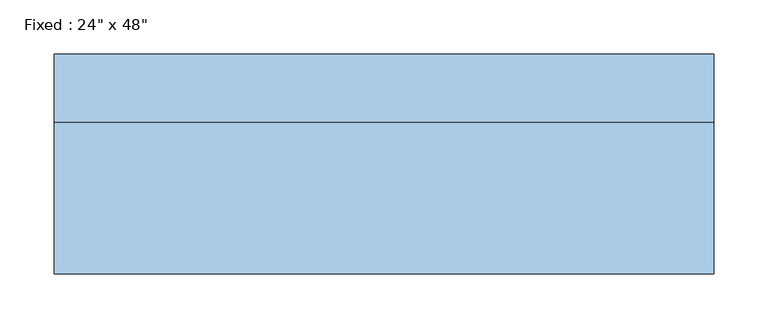
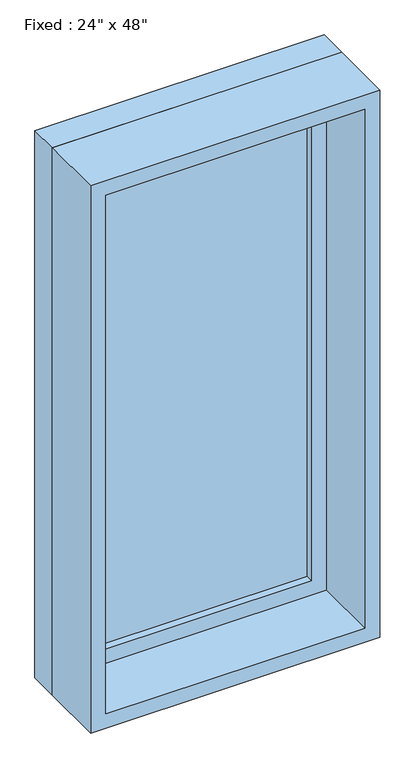
"""IFC4 building model written with IfcOpenShell, lengths in millimetres: window geometry."""

from ifc_helpers import new_model, si_unit, frame, origin, place, context, project, spatial, polyline, outline, extrude, source, transform, mapped, element, save


def window_80bd9af0(model_context):
    return source(origin(), model_context, "Body", "SweptSolid", [
        extrude(outline(polyline([(203.2, 53.975), (-279.4, 53.975), (-279.4, 66.675), (203.2, 66.675), (203.2, 53.975)])), frame((0.0, 0.0, 977.9), z_axis=(0.0, 0.0, 1.0), x_axis=(1.0, 0.0, 0.0)), (0.0, 0.0, 1.0), 1092.2),
        extrude(outline(polyline([(2114.55, -323.85), (933.45, -323.85), (933.45, 247.65), (2114.55, 247.65), (2114.55, -323.85)]), holes=[polyline([(2070.1, -279.4), (2070.1, 203.2), (977.9, 203.2), (977.9, -279.4), (2070.1, -279.4)])]), frame((0.0, 38.1, 0.0), z_axis=(0.0, 1.0, 0.0), x_axis=(0.0, 0.0, 1.0)), (0.0, 0.0, 1.0), 44.45),
        extrude(outline(polyline([(2133.6, -342.9), (914.4, -342.9), (914.4, 266.7), (2133.6, 266.7), (2133.6, -342.9)]), holes=[polyline([(2101.85, -311.15), (2101.85, 234.95), (946.15, 234.95), (946.15, -311.15), (2101.85, -311.15)])]), frame((0.0, -101.6, 0.0), z_axis=(0.0, 1.0, 0.0), x_axis=(0.0, 0.0, 1.0)), (0.0, 0.0, 1.0), 139.7),
        extrude(outline(polyline([(2133.6, 266.7), (2133.6, -342.9), (914.4, -342.9), (914.4, 266.7), (2133.6, 266.7)]), holes=[polyline([(2114.55, 247.65), (933.45, 247.65), (933.45, -323.85), (2114.55, -323.85), (2114.55, 247.65)])]), frame((0.0, 38.1, 0.0), z_axis=(0.0, 1.0, 0.0), x_axis=(0.0, 0.0, 1.0)), (0.0, 0.0, 1.0), 63.5),
    ])


if __name__ == "__main__":
    model = new_model("IFC4")
    model_context = context("Model", 3, world=origin())
    ifc_project = project(units=[si_unit("LENGTHUNIT", "METRE", prefix="MILLI")], contexts=[model_context])
    site = spatial("IfcSite", under=ifc_project)
    building = spatial("IfcBuilding", under=site)
    placement = place(None, origin())
    window_shape = window_80bd9af0(model_context)
    element("IfcWindow", 1, ObjectType="Fixed : 24\" x 48\"", at=placement, inside=building, context=model_context, shape_type="MappedRepresentation", body=[
        mapped(window_shape, transform((0.0, 0.0, 0.0), x_axis=(1.0, 0.0, 0.0), y_axis=(0.0, 1.0, 0.0), z_axis=(0.0, 0.0, 1.0))),
    ])
    save(model, "model.ifc")

# Revit data of these elements
# Type "Fixed : 24\" x 48\""
#   Type Mark = "2"
#   Construction Type Id = "GSP4R"
#   Assembly Code = "B2020100"
#   Analytic Construction = "1/8 in Pilkington single glazing"
#   Visual Light Transmittance = 0.9
#   Solar Heat Gain Coefficient = 0.78
#   Heat Transfer Coefficient (U) = 0.6496 BTU/(h·ft²·°F)
#   Height = 4' - 0"
#   Default Sill Height = 3' - 0"
#   Width = 2' - 0"
#   Window Inset = 0' - 0 3/4"
#   Define Thermal Properties by = 1
#   Glass Pane Material = Glass
#   Sash Material = Sash
#   Wall Closure = (empty or 0)
# Element 1 (IfcWindow, "Fixed : 24\" x 48\"")
#   Materials on its faces: "Sash", "Glass"
# Materials
#   "Glass": class "Glass", colour RGB 0 128 192, transparency 0.75, Description = "Soda Lime Glass", Cost = 0
#   "Sash": class "Wood", colour RGB 224 178 126, transparency 0
